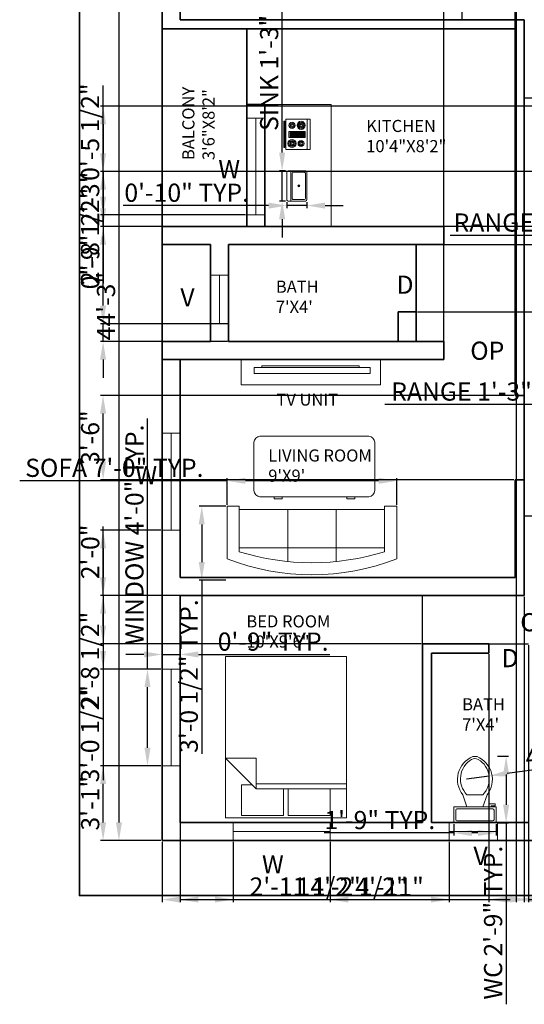
# Model space of a CAD drawing. Units: inches. Extents: x 53076 to 53578, y 41072 to 41816.
# Tile 1 of 4: x 53076 to 53326, y 41072 to 41560. Entities that reach past the tile are written whole.
import ezdxf

# ---------------------------------------------------------------- set-up
doc = ezdxf.new("R2010")
doc.units = ezdxf.units.IN
for name, color, linetype, lineweight in [('A-ANNO-DIMS', 2, 'Continuous', 18), ('A-ANNO-TEXT', 7, 'Continuous', 18), ('A-ANNO-TTLB', 7, 'Continuous', 35), ('A-AREA-IDEN', 7, 'Continuous', 18), ('A-DOOR', 3, 'Continuous', 25), ('A-EQPM', 8, 'Continuous', 18), ('A-FLOR-CASE', 9, 'Continuous', 18), ('A-FLOR-FIXT', 9, 'Continuous', 18), ('A-FURN', 8, 'Continuous', 18), ('A-GLAZ', 4, 'Continuous', 18), ('A-WALL', 7, 'Continuous', 35)]:
    doc.layers.add(name, color=color, linetype=linetype, lineweight=lineweight)
doc.styles.get("Standard").update_dxf_attribs({"font": 'arial.ttf'})
doc.dimstyles.new('ISO-25', dxfattribs={"dimtxt": 9, "dimasz": 9, "dimexe": 1.25, "dimexo": 0.625, "dimtad": 1, "dimdec": 1, "dimrnd": 9, "dimlunit": 3, "dimtxsty": 'Standard', "dimcen": 2.5, "dimadec": 0, "dimazin": 0, "dimtfac": 1, "dimtdec": 1, "dimtmove": 0, "dimatfit": 3, "dimfxl": 1, "dimarcsym": 0})

# ---------------------------------------------------------------- blocks, each defined once
blk = doc.blocks.new('*D2')
at = {"layer": 'A-ANNO-DIMS', "color": 0, "lineweight": -2, "transparency": 16777216}
for p, q in [((53146.18, 41682.66), (53124.21, 41682.66)), ((53125.46, 41673.66), (53125.46, 41161.66)), ((53146.18, 41152.66), (53124.21, 41152.66))]:
    blk.add_line(p, q, dxfattribs=at)
at = {"layer": 'A-ANNO-DIMS', "color": 0, "transparency": 16777216}
for points in [[(53123.96, 41673.66), (53126.96, 41673.66), (53125.46, 41682.66)], [(53123.96, 41161.66), (53126.96, 41161.66), (53125.46, 41152.66)]]:
    blk.add_solid(points, dxfattribs=at)
at = {"layer": 'Defpoints', "color": 0, "transparency": 16777216}
for p in [(53146.81, 41682.66), (53125.46, 41152.66), (53146.81, 41152.66)]:
    blk.add_point(p, dxfattribs=at)
at = {"layer": 'A-ANNO-DIMS', "color": 0, "transparency": 16777216, "insert": (53120.23, 41417.66), "char_height": 9, "attachment_point": 5, "rotation": 90}
blk.add_mtext('44\'-3"', dxfattribs=at)
blk = doc.blocks.new('Range-Oven - 30 in top')
for p, q in [((0, -3), (30, -3)), ((12, -6), (18, -6)), ((13, -20), (13, -6)), ((14, -6), (14, -20)), ((15, -20), (15, -6)), ((16, -6), (16, -20)), ((17, -20), (17, -6)), ((6, -24), (6, -25)), ((8, -25), (8, -24)), ((18, -20), (12, -20)), ((22, -25), (22, -24)), ((24, -24), (24, -25))]:
    blk.add_line(p, q)
for points in [[(0, -24), (0, 0), (30, 0), (30, -24)], [(12, -21), (12, -5), (18, -5), (18, -21)], [(2, -26), (2, -25), (28, -25), (28, -26)]]:
    blk.add_lwpolyline(points, close=True)
for centre, radius in [((6, -9), 4), ((6, -9), 3), ((6, -9), 2), ((6, -9), 1), ((24, -9), 3), ((24, -9), 2), ((24, -9), 1), ((6, -18), 3), ((6, -18), 2), ((6, -18), 1), ((24, -18), 4), ((24, -18), 3), ((24, -18), 2), ((24, -18), 1)]:
    blk.add_circle(centre, radius)
blk = doc.blocks.new('Sink-single - 30 in top')
blk.add_line((-15, -3.999996), (15, -3.999996))
for points in [[(-13.5, 0), (13.5, 0)], [(-15, -18.499996), (-15, -1.5)], [(-13.5, -17.499996), (-13.5, -6.499996)], [(-12.5, -5.499996), (12.5, -5.499996)], [(13.5, -6.499996), (13.5, -17.499996)], [(15, -1.5), (15, -18.499996)], [(12.5, -18.499996), (-12.5, -18.499996)], [(13.5, -19.999996), (-13.5, -19.999996)]]:
    blk.add_lwpolyline(points)
for radius in [1, 0.5]:
    blk.add_circle((0, -11.999996), radius)
for centre, radius, start, end in [((-13.5, -1.5), 1.5, 90, 180), ((-12.5, -6.499996), 1, 90, 180), ((12.5, -6.499996), 1, 0, 90), ((13.5, -1.5), 1.5, 0, 90), ((-13.5, -18.499996), 1.5, 180, 270), ((-12.5, -17.499996), 1, 180, 270), ((12.5, -17.499996), 1, 270, 0), ((13.5, -18.499996), 1.5, 270, 0)]:
    blk.add_arc(centre, radius, start, end)
blk = doc.blocks.new('Sofa - Roundback 7 ft.')
for p, q in [((-12.00002, -32.4421), (-12.00003, -6.5971)), ((11.99997, -32.4421), (11.99998, -6.5971)), ((-36.000027, -34), (-36.000027, -11.4696)), ((-35.999844, -13.3819), (35.9998, -13.3819)), ((35.99998, -34), (35.99998, -11.4696)), ((-36.000027, -32.4421), (35.99998, -32.4421))]:
    blk.add_line(p, q)
for points in [[(-36.000027, -34), (-42.000027, -34), (-42.000027, -8)], [(41.99998, -8), (41.99998, -34), (35.99998, -34)]]:
    blk.add_lwpolyline(points)
for centre, radius, start, end in [((0, -114.25), 114.25, 68.43141, 111.5686), ((-0.00001, -127.1968), 121.1968, 72.72033, 107.2797)]:
    blk.add_arc(centre, radius, start, end)
blk = doc.blocks.new('Desk - 30 x 60 in.')
for p, q in [((-26.999995, 0), (26.999995, 0)), ((-29.999995, -27), (-29.999995, -3)), ((29.999995, -3), (29.999995, -27)), ((26.999995, -30), (-26.999995, -30)), ((-20.000005, -30), (-20.000005, -31)), ((-20.000005, -31), (-16.000005, -31)), ((-16.000005, -31), (-16.000005, -30)), ((15.999995, -31), (15.999995, -30)), ((19.999995, -31), (15.999995, -31)), ((19.999995, -30), (19.999995, -31))]:
    blk.add_line(p, q)
for centre, start, end in [((-26.499995, -3.5), 98.1301, 171.8699), ((26.499995, -3.5), 8.130102, 81.8699), ((-26.499995, -26.5), 188.1301, 261.8699), ((26.499995, -26.5), 278.1301, 351.8699)]:
    blk.add_arc(centre, 3.535534, start, end)
blk = doc.blocks.new('Bed - Queen')
for p, q in [((0, -80.00003), (0, 0)), ((0, 0), (59.99999, 0)), ((59.99999, 0), (59.99999, -80.00003)), ((7.99999, -1.2), (28.79998, -1.2)), ((7.99999, -14.4), (7.99999, -1.2)), ((28.79998, -1.2), (28.79998, -14.4)), ((31.19999, -1.2), (51.99999, -1.2)), ((31.19999, -14.4), (31.19999, -1.2)), ((51.99999, -1.2), (51.99999, -16.4)), ((0, -14.4), (44.8, -14.4)), ((59.99999, -29.6), (44.8, -14.4)), ((44.8, -14.4), (44.8, -29.6)), ((44.8, -16.8), (0, -16.8)), ((51.99999, -16.4), (46.79936, -16.4)), ((44.8, -29.6), (59.99999, -29.6)), ((59.99999, -80.00003), (0, -80.00003))]:
    blk.add_line(p, q)
blk = doc.blocks.new('Toilet - top')
for p, q in [((9.5, -6), (9.5, -2)), ((-10, -8.5), (-8, -8.5)), ((-10, -9.5), (-10, -8.5)), ((-7, -9.5), (-10, -9.5)), ((-8, -8.5), (-8, -8)), ((-7, -8), (-7, -9.5)), ((-4, -8), (-6, -14)), ((4, -8), (6, -14)), ((4, -14), (-4, -14))]:
    blk.add_line(p, q)
blk.add_lwpolyline([(10.5, -8), (10.5, 0), (-10.5, 0), (-10.5, -8)], close=True)
for points in [[(-9.5, -2), (-9.5, -6)], [(8.5, -1), (-8.5, -1)], [(-8.5, -7), (8.5, -7)]]:
    blk.add_lwpolyline(points)
for centre, radius, start, end in [((-8.62, -1.88), 0.884, 81.8699, 188.1301), ((8.62, -1.88), 0.884, 351.8699, 98.1301), ((-8.62, -6.12), 0.884, 171.8699, 278.1301), ((8.62, -6.12), 0.884, 261.8699, 8.1301), ((3.52, -21.58), 12.17, 141.4691, 247.9714), ((4.2, -21.82), 11.33, 136.3677, 238.9468), ((-3.52, -21.58), 12.17, 292.0284, 38.5307), ((-4.2, -21.82), 11.33, 301.053, 43.6321), ((0, -27.88), 4, 245.7318, 294.2682), ((0, -29), 4, 254.8605, 285.1395)]:
    blk.add_arc(centre, radius, start, end)
blk = doc.blocks.new('WIN-48IN')
for p, q in [((0, 48), (9, 48)), ((4.5, 48), (4.5, 0)), ((0, 0), (9, 0))]:
    blk.add_line(p, q)
blk = doc.blocks.new('VENT-24IN')
for p, q in [((0, 9), (0, 0)), ((24, 9), (24, 0)), ((0, 4.5), (24, 4.5))]:
    blk.add_line(p, q)
blk = doc.blocks.new('DOOR-ENTRY-28_5IN')
blk.add_line((0, 0), (28.5, 0))
blk = doc.blocks.new('*D12')
at = {"layer": 'A-ANNO-DIMS', "color": 0, "lineweight": -2, "transparency": 16777216}
for p, q in [((53139.61, 41237.75), (53139.61, 41361.89)), ((53146.18, 41237.75), (53138.36, 41237.75)), ((53139.61, 41198.75), (53139.61, 41228.75)), ((53146.18, 41189.75), (53138.36, 41189.75))]:
    blk.add_line(p, q, dxfattribs=at)
at = {"layer": 'A-ANNO-DIMS', "color": 0, "transparency": 16777216}
for points in [[(53138.11, 41228.75), (53141.11, 41228.75), (53139.61, 41237.75)], [(53138.11, 41198.75), (53141.11, 41198.75), (53139.61, 41189.75)]]:
    blk.add_solid(points, dxfattribs=at)
at = {"layer": 'Defpoints', "color": 0, "transparency": 16777216}
for p in [(53139.61, 41237.75), (53146.81, 41237.75), (53146.81, 41189.75)]:
    blk.add_point(p, dxfattribs=at)
at = {"layer": 'A-ANNO-DIMS', "color": 0, "transparency": 16777216, "insert": (53134.32, 41304.32), "char_height": 9, "attachment_point": 5, "rotation": 90}
blk.add_mtext('WINDOW 4\'-0" TYP.', dxfattribs=at)
blk = doc.blocks.new('*D13')
at = {"layer": 'A-ANNO-DIMS', "color": 0, "lineweight": -2, "transparency": 16777216}
for p, q in [((53137.81, 41244.95), (53128.81, 41244.95)), ((53146.81, 41238.38), (53146.81, 41246.2)), ((53146.81, 41244.95), (53155.81, 41244.95)), ((53155.81, 41238.38), (53155.81, 41246.2)), ((53164.81, 41244.95), (53229.92, 41244.95))]:
    blk.add_line(p, q, dxfattribs=at)
at = {"layer": 'A-ANNO-DIMS', "color": 0, "transparency": 16777216}
for points in [[(53137.81, 41246.45), (53137.81, 41243.45), (53146.81, 41244.95)], [(53164.81, 41246.45), (53164.81, 41243.45), (53155.81, 41244.95)]]:
    blk.add_solid(points, dxfattribs=at)
at = {"layer": 'Defpoints', "color": 0, "transparency": 16777216}
for p in [(53155.81, 41244.95), (53146.81, 41237.75), (53155.81, 41237.75)]:
    blk.add_point(p, dxfattribs=at)
at = {"layer": 'A-ANNO-DIMS', "color": 0, "transparency": 16777216, "insert": (53201.86, 41250.17), "char_height": 9, "attachment_point": 5}
blk.add_mtext('0\'-9" TYP.', dxfattribs=at)
blk = doc.blocks.new('*D14')
at = {"layer": 'A-ANNO-DIMS', "color": 0, "lineweight": -2, "transparency": 16777216}
for p, q in [((53179.09, 41331.04), (53076.3, 41331.04)), ((53179.09, 41319.06), (53179.09, 41332.29)), ((53254.09, 41331.04), (53188.09, 41331.04)), ((53263.09, 41319.06), (53263.09, 41332.29))]:
    blk.add_line(p, q, dxfattribs=at)
at = {"layer": 'A-ANNO-DIMS', "color": 0, "transparency": 16777216}
for points in [[(53188.09, 41332.54), (53188.09, 41329.54), (53179.09, 41331.04)], [(53254.09, 41332.54), (53254.09, 41329.54), (53263.09, 41331.04)]]:
    blk.add_solid(points, dxfattribs=at)
at = {"layer": 'Defpoints', "color": 0, "transparency": 16777216}
for p in [(53179.09, 41331.04), (53179.09, 41318.44), (53263.09, 41318.44)]:
    blk.add_point(p, dxfattribs=at)
at = {"layer": 'A-ANNO-DIMS', "color": 0, "transparency": 16777216, "insert": (53123.19, 41336.32), "char_height": 9, "attachment_point": 5}
blk.add_mtext('SOFA 7\'-0" TYP.', dxfattribs=at)
blk = doc.blocks.new('*D15')
at = {"layer": 'A-ANNO-DIMS', "color": 0, "lineweight": -2, "transparency": 16777216}
for p, q in [((53178.46, 41318.44), (53165.24, 41318.44)), ((53166.49, 41309.44), (53166.49, 41290.77)), ((53178.46, 41281.77), (53165.24, 41281.77)), ((53166.49, 41281.77), (53166.49, 41195.7))]:
    blk.add_line(p, q, dxfattribs=at)
at = {"layer": 'A-ANNO-DIMS', "color": 0, "transparency": 16777216}
for points in [[(53164.99, 41309.44), (53167.99, 41309.44), (53166.49, 41318.44)], [(53164.99, 41290.77), (53167.99, 41290.77), (53166.49, 41281.77)]]:
    blk.add_solid(points, dxfattribs=at)
at = {"layer": 'Defpoints', "color": 0, "transparency": 16777216}
for p in [(53179.09, 41318.44), (53166.49, 41281.77), (53179.09, 41281.77)]:
    blk.add_point(p, dxfattribs=at)
at = {"layer": 'A-ANNO-DIMS', "color": 0, "transparency": 16777216, "insert": (53161.21, 41234.23), "char_height": 9, "attachment_point": 5, "rotation": 90}
blk.add_mtext('3\'-0 1/2" TYP.', dxfattribs=at)
blk = doc.blocks.new('*D18')
at = {"layer": 'A-ANNO-DIMS', "color": 0, "lineweight": -2, "transparency": 16777216}
for p, q in [((53206.33, 41493.74), (53206.33, 41591.64)), ((53207.95, 41484.74), (53205.08, 41484.74)), ((53206.33, 41469.74), (53206.33, 41484.74)), ((53207.95, 41469.74), (53205.08, 41469.74)), ((53206.33, 41460.74), (53206.33, 41451.74))]:
    blk.add_line(p, q, dxfattribs=at)
at = {"layer": 'A-ANNO-DIMS', "color": 0, "transparency": 16777216}
for points in [[(53204.83, 41493.74), (53207.83, 41493.74), (53206.33, 41484.74)], [(53204.83, 41460.74), (53207.83, 41460.74), (53206.33, 41469.74)]]:
    blk.add_solid(points, dxfattribs=at)
at = {"layer": 'Defpoints', "color": 0, "transparency": 16777216}
for p in [(53206.33, 41484.74), (53208.58, 41484.74), (53208.58, 41469.74)]:
    blk.add_point(p, dxfattribs=at)
at = {"layer": 'A-ANNO-DIMS', "color": 0, "transparency": 16777216, "insert": (53201.05, 41547.19), "char_height": 9, "attachment_point": 5, "rotation": 90}
blk.add_mtext('SINK 1\'-3" TYP.', dxfattribs=at)
blk = doc.blocks.new('*D19')
at = {"layer": 'A-ANNO-DIMS', "color": 0, "lineweight": -2, "transparency": 16777216}
for p, q in [((53199.58, 41467.49), (53127.48, 41467.49)), ((53208.58, 41469.11), (53208.58, 41466.24)), ((53218.58, 41467.49), (53208.58, 41467.49)), ((53218.58, 41469.11), (53218.58, 41466.24)), ((53227.58, 41467.49), (53236.58, 41467.49))]:
    blk.add_line(p, q, dxfattribs=at)
at = {"layer": 'A-ANNO-DIMS', "color": 0, "transparency": 16777216}
for points in [[(53199.58, 41468.99), (53199.58, 41465.99), (53208.58, 41467.49)], [(53227.58, 41468.99), (53227.58, 41465.99), (53218.58, 41467.49)]]:
    blk.add_solid(points, dxfattribs=at)
at = {"layer": 'Defpoints', "color": 0, "transparency": 16777216}
for p in [(53208.58, 41469.74), (53208.58, 41467.49), (53218.58, 41469.74)]:
    blk.add_point(p, dxfattribs=at)
at = {"layer": 'A-ANNO-DIMS', "color": 0, "transparency": 16777216, "insert": (53159.03, 41472.71), "char_height": 9, "attachment_point": 5}
blk.add_mtext('0\'-10" TYP.', dxfattribs=at)
blk = doc.blocks.new('*D20')
at = {"layer": 'A-ANNO-DIMS', "color": 0, "lineweight": -2, "transparency": 16777216}
for p, q in [((53371.57, 41452.66), (53289.65, 41452.66)), ((53371.57, 41456.53), (53371.57, 41451.41)), ((53392.57, 41452.66), (53380.57, 41452.66)), ((53401.57, 41456.53), (53401.57, 41451.41))]:
    blk.add_line(p, q, dxfattribs=at)
at = {"layer": 'A-ANNO-DIMS', "color": 0, "transparency": 16777216}
for points in [[(53380.57, 41454.16), (53380.57, 41451.16), (53371.57, 41452.66)], [(53392.57, 41454.16), (53392.57, 41451.16), (53401.57, 41452.66)]]:
    blk.add_solid(points, dxfattribs=at)
at = {"layer": 'Defpoints', "color": 0, "transparency": 16777216}
for p in [(53371.57, 41457.16), (53371.57, 41452.66), (53401.57, 41457.16)]:
    blk.add_point(p, dxfattribs=at)
at = {"layer": 'A-ANNO-DIMS', "color": 0, "transparency": 16777216, "insert": (53326.11, 41457.93), "char_height": 9, "attachment_point": 5}
blk.add_mtext('RANGE 2\'-6"', dxfattribs=at)
blk = doc.blocks.new('*D22')
at = {"layer": 'A-ANNO-DIMS', "color": 0, "lineweight": -2, "transparency": 16777216}
for p, q in [((53379.04, 41367.23), (53379.04, 41370.11)), ((53394.04, 41367.23), (53394.04, 41370.11)), ((53370.04, 41368.86), (53257.19, 41368.86)), ((53394.04, 41368.86), (53379.04, 41368.86)), ((53403.04, 41368.86), (53412.04, 41368.86))]:
    blk.add_line(p, q, dxfattribs=at)
at = {"layer": 'A-ANNO-DIMS', "color": 0, "transparency": 16777216}
for points in [[(53370.04, 41370.36), (53370.04, 41367.36), (53379.04, 41368.86)], [(53403.04, 41370.36), (53403.04, 41367.36), (53394.04, 41368.86)]]:
    blk.add_solid(points, dxfattribs=at)
at = {"layer": 'Defpoints', "color": 0, "transparency": 16777216}
for p in [(53379.04, 41368.86), (53379.04, 41366.61), (53394.04, 41366.61)]:
    blk.add_point(p, dxfattribs=at)
at = {"layer": 'A-ANNO-DIMS', "color": 0, "transparency": 16777216, "insert": (53309.12, 41374.14), "char_height": 9, "attachment_point": 5}
blk.add_mtext('RANGE 1\'-3" TYP.', dxfattribs=at)
blk = doc.blocks.new('*D30')
at = {"layer": 'A-ANNO-DIMS', "color": 0, "lineweight": -2, "transparency": 16777216}
for p, q in [((53312.97, 41194.48), (53318.55, 41194.48)), ((53317.3, 41185.48), (53317.3, 41170.44)), ((53312.97, 41161.44), (53318.55, 41161.44)), ((53317.3, 41161.44), (53317.3, 41071.52))]:
    blk.add_line(p, q, dxfattribs=at)
at = {"layer": 'A-ANNO-DIMS', "color": 0, "transparency": 16777216}
for points in [[(53315.8, 41185.48), (53318.8, 41185.48), (53317.3, 41194.48)], [(53315.8, 41170.44), (53318.8, 41170.44), (53317.3, 41161.44)]]:
    blk.add_solid(points, dxfattribs=at)
at = {"layer": 'Defpoints', "color": 0, "transparency": 16777216}
for p in [(53312.34, 41194.48), (53312.34, 41161.44), (53317.3, 41161.44)]:
    blk.add_point(p, dxfattribs=at)
at = {"layer": 'A-ANNO-DIMS', "color": 0, "transparency": 16777216, "insert": (53312.02, 41111.98), "char_height": 9, "attachment_point": 5, "rotation": 90}
blk.add_mtext('WC 2\'-9" TYP.', dxfattribs=at)
blk = doc.blocks.new('*D31')
at = {"layer": 'A-ANNO-DIMS', "color": 0, "lineweight": -2, "transparency": 16777216}
for p, q in [((53291.34, 41160.81), (53291.34, 41155.23)), ((53312.34, 41160.81), (53312.34, 41155.23)), ((53291.34, 41156.48), (53227.08, 41156.48)), ((53303.34, 41156.48), (53300.34, 41156.48))]:
    blk.add_line(p, q, dxfattribs=at)
at = {"layer": 'A-ANNO-DIMS', "color": 0, "transparency": 16777216}
for points in [[(53300.34, 41157.98), (53300.34, 41154.98), (53291.34, 41156.48)], [(53303.34, 41157.98), (53303.34, 41154.98), (53312.34, 41156.48)]]:
    blk.add_solid(points, dxfattribs=at)
at = {"layer": 'Defpoints', "color": 0, "transparency": 16777216}
for p in [(53291.34, 41161.44), (53312.34, 41161.44), (53291.34, 41156.48)]:
    blk.add_point(p, dxfattribs=at)
at = {"layer": 'A-ANNO-DIMS', "color": 0, "transparency": 16777216, "insert": (53254.71, 41161.7), "char_height": 9, "attachment_point": 5}
blk.add_mtext('1\'-9" TYP.', dxfattribs=at)
blk = doc.blocks.new('*D36')
at = {"layer": 'A-ANNO-DIMS', "color": 0, "lineweight": -2, "transparency": 16777216}
for p, q in [((53155.18, 41274.16), (53116.36, 41274.16)), ((53117.61, 41265.16), (53117.61, 41246.75)), ((53146.18, 41237.75), (53116.36, 41237.75)), ((53117.61, 41237.75), (53117.61, 41182.61))]:
    blk.add_line(p, q, dxfattribs=at)
at = {"layer": 'A-ANNO-DIMS', "color": 0, "transparency": 16777216}
for points in [[(53116.11, 41265.16), (53119.11, 41265.16), (53117.61, 41274.16)], [(53116.11, 41246.75), (53119.11, 41246.75), (53117.61, 41237.75)]]:
    blk.add_solid(points, dxfattribs=at)
at = {"layer": 'Defpoints', "color": 0, "transparency": 16777216}
for p in [(53155.81, 41274.16), (53117.61, 41237.75), (53146.81, 41237.75)]:
    blk.add_point(p, dxfattribs=at)
at = {"layer": 'A-ANNO-DIMS', "color": 0, "transparency": 16777216, "insert": (53112.32, 41205.68), "char_height": 9, "attachment_point": 5, "rotation": 90}
blk.add_mtext('3\'-0 1/2"', dxfattribs=at)
blk = doc.blocks.new('*D42')
at = {"layer": 'A-ANNO-DIMS', "color": 0, "lineweight": -2, "transparency": 16777216}
for p, q in [((53146.81, 41152.03), (53146.81, 41122.21)), ((53182.09, 41152.03), (53182.09, 41122.21)), ((53155.81, 41123.46), (53173.09, 41123.46)), ((53182.09, 41123.46), (53244.38, 41123.46))]:
    blk.add_line(p, q, dxfattribs=at)
at = {"layer": 'A-ANNO-DIMS', "color": 0, "transparency": 16777216}
for points in [[(53155.81, 41124.96), (53155.81, 41121.96), (53146.81, 41123.46)], [(53173.09, 41124.96), (53173.09, 41121.96), (53182.09, 41123.46)]]:
    blk.add_solid(points, dxfattribs=at)
at = {"layer": 'Defpoints', "color": 0, "transparency": 16777216}
for p in [(53146.81, 41152.66), (53182.09, 41152.66), (53182.09, 41123.46)]:
    blk.add_point(p, dxfattribs=at)
at = {"layer": 'A-ANNO-DIMS', "color": 0, "transparency": 16777216, "insert": (53217.73, 41128.73), "char_height": 9, "attachment_point": 5}
blk.add_mtext('2\'-11 1/2"', dxfattribs=at)
blk = doc.blocks.new('*D43')
at = {"layer": 'A-ANNO-DIMS', "color": 0, "lineweight": -2, "transparency": 16777216}
for p, q in [((53230.09, 41152.03), (53230.09, 41122.21)), ((53289.01, 41152.03), (53289.01, 41122.21)), ((53239.09, 41123.46), (53280.01, 41123.46))]:
    blk.add_line(p, q, dxfattribs=at)
at = {"layer": 'A-ANNO-DIMS', "color": 0, "transparency": 16777216}
for points in [[(53239.09, 41124.96), (53239.09, 41121.96), (53230.09, 41123.46)], [(53280.01, 41124.96), (53280.01, 41121.96), (53289.01, 41123.46)]]:
    blk.add_solid(points, dxfattribs=at)
at = {"layer": 'Defpoints', "color": 0, "transparency": 16777216}
for p in [(53230.09, 41152.66), (53289.01, 41152.66), (53289.01, 41123.46)]:
    blk.add_point(p, dxfattribs=at)
at = {"layer": 'A-ANNO-DIMS', "color": 0, "transparency": 16777216, "insert": (53259.55, 41128.6), "char_height": 9, "attachment_point": 5}
blk.add_mtext('4\'-11"', dxfattribs=at)
blk = doc.blocks.new('*D46')
at = {"layer": 'A-ANNO-DIMS', "color": 0, "lineweight": -2, "transparency": 16777216}
for p, q in [((53146.18, 41306.6), (53116.36, 41306.6)), ((53117.61, 41297.6), (53117.61, 41283.16)), ((53155.18, 41274.16), (53116.36, 41274.16)), ((53117.61, 41274.16), (53117.61, 41218.86))]:
    blk.add_line(p, q, dxfattribs=at)
at = {"layer": 'A-ANNO-DIMS', "color": 0, "transparency": 16777216}
for points in [[(53116.11, 41297.6), (53119.11, 41297.6), (53117.61, 41306.6)], [(53116.11, 41283.16), (53119.11, 41283.16), (53117.61, 41274.16)]]:
    blk.add_solid(points, dxfattribs=at)
at = {"layer": 'Defpoints', "color": 0, "transparency": 16777216}
for p in [(53146.81, 41306.6), (53117.61, 41274.16), (53155.81, 41274.16)]:
    blk.add_point(p, dxfattribs=at)
at = {"layer": 'A-ANNO-DIMS', "color": 0, "transparency": 16777216, "insert": (53112.33, 41242.01), "char_height": 9, "attachment_point": 5, "rotation": 90}
blk.add_mtext('2\'-8 1/2"', dxfattribs=at)
blk = doc.blocks.new('*D47')
at = {"layer": 'A-ANNO-DIMS', "color": 0, "lineweight": -2, "transparency": 16777216}
for p, q in [((53146.18, 41189.75), (53116.36, 41189.75)), ((53117.61, 41161.66), (53117.61, 41180.75)), ((53146.18, 41152.66), (53116.36, 41152.66))]:
    blk.add_line(p, q, dxfattribs=at)
at = {"layer": 'A-ANNO-DIMS', "color": 0, "transparency": 16777216}
for points in [[(53116.11, 41180.75), (53119.11, 41180.75), (53117.61, 41189.75)], [(53116.11, 41161.66), (53119.11, 41161.66), (53117.61, 41152.66)]]:
    blk.add_solid(points, dxfattribs=at)
at = {"layer": 'Defpoints', "color": 0, "transparency": 16777216}
for p in [(53117.61, 41189.75), (53146.81, 41189.75), (53146.81, 41152.66)]:
    blk.add_point(p, dxfattribs=at)
at = {"layer": 'A-ANNO-DIMS', "color": 0, "transparency": 16777216, "insert": (53112.38, 41171.2), "char_height": 9, "attachment_point": 5, "rotation": 90}
blk.add_mtext('3\'-1"', dxfattribs=at)
blk = doc.blocks.new('*D50')
at = {"layer": 'A-ANNO-DIMS', "color": 0, "lineweight": -2, "transparency": 16777216}
for p, q in [((53117.61, 41471.84), (53117.61, 41526.99)), ((53188.18, 41462.84), (53116.36, 41462.84)), ((53117.61, 41457.16), (53117.61, 41462.84)), ((53188.18, 41457.16), (53116.36, 41457.16)), ((53117.61, 41448.16), (53117.61, 41439.16))]:
    blk.add_line(p, q, dxfattribs=at)
at = {"layer": 'A-ANNO-DIMS', "color": 0, "transparency": 16777216}
for points in [[(53116.11, 41471.84), (53119.11, 41471.84), (53117.61, 41462.84)], [(53116.11, 41448.16), (53119.11, 41448.16), (53117.61, 41457.16)]]:
    blk.add_solid(points, dxfattribs=at)
at = {"layer": 'Defpoints', "color": 0, "transparency": 16777216}
for p in [(53117.61, 41462.84), (53188.81, 41462.84), (53188.81, 41457.16)]:
    blk.add_point(p, dxfattribs=at)
at = {"layer": 'A-ANNO-DIMS', "color": 0, "transparency": 16777216, "insert": (53112.33, 41503.92), "char_height": 9, "attachment_point": 5, "rotation": 90}
blk.add_mtext('0\'-5 1/2"', dxfattribs=at)
blk = doc.blocks.new('*D51')
at = {"layer": 'A-ANNO-DIMS', "color": 0, "lineweight": -2, "transparency": 16777216}
for p, q in [((53117.61, 41417.95), (53117.61, 41452.12)), ((53179.18, 41408.95), (53116.36, 41408.95)), ((53117.61, 41400.16), (53117.61, 41408.95)), ((53179.18, 41400.16), (53116.36, 41400.16)), ((53117.61, 41391.16), (53117.61, 41382.16))]:
    blk.add_line(p, q, dxfattribs=at)
at = {"layer": 'A-ANNO-DIMS', "color": 0, "transparency": 16777216}
for points in [[(53116.11, 41417.95), (53119.11, 41417.95), (53117.61, 41408.95)], [(53116.11, 41391.16), (53119.11, 41391.16), (53117.61, 41400.16)]]:
    blk.add_solid(points, dxfattribs=at)
at = {"layer": 'Defpoints', "color": 0, "transparency": 16777216}
for p in [(53117.61, 41408.95), (53179.81, 41408.95), (53179.81, 41400.16)]:
    blk.add_point(p, dxfattribs=at)
at = {"layer": 'A-ANNO-DIMS', "color": 0, "transparency": 16777216, "insert": (53112.39, 41439.54), "char_height": 9, "attachment_point": 5, "rotation": 90}
blk.add_mtext('0\'-9"', dxfattribs=at)
blk = doc.blocks.new('*D55')
at = {"layer": 'A-ANNO-DIMS', "color": 0, "lineweight": -2, "transparency": 16777216}
for p, q in [((53322.2, 41589.03), (53322.2, 41122.21)), ((53343.31, 41584.53), (53343.31, 41122.21)), ((53331.2, 41123.46), (53334.31, 41123.46)), ((53343.31, 41123.46), (53376.63, 41123.46))]:
    blk.add_line(p, q, dxfattribs=at)
at = {"layer": 'A-ANNO-DIMS', "color": 0, "transparency": 16777216}
for points in [[(53331.2, 41124.96), (53331.2, 41121.96), (53322.2, 41123.46)], [(53334.31, 41124.96), (53334.31, 41121.96), (53343.31, 41123.46)]]:
    blk.add_solid(points, dxfattribs=at)
at = {"layer": 'Defpoints', "color": 0, "transparency": 16777216}
for p in [(53322.2, 41589.66), (53343.31, 41585.16), (53343.31, 41123.46)]:
    blk.add_point(p, dxfattribs=at)
at = {"layer": 'A-ANNO-DIMS', "color": 0, "transparency": 16777216, "insert": (53364.47, 41128.68), "char_height": 9, "attachment_point": 5}
blk.add_mtext('1\'-9"', dxfattribs=at)
blk = doc.blocks.new('*D57')
at = {"layer": 'A-ANNO-DIMS', "color": 0, "lineweight": -2, "transparency": 16777216}
for p, q in [((53321.18, 41373.39), (53116.36, 41373.39)), ((53117.61, 41340.53), (53117.61, 41364.39)), ((53321.18, 41331.53), (53116.36, 41331.53))]:
    blk.add_line(p, q, dxfattribs=at)
at = {"layer": 'A-ANNO-DIMS', "color": 0, "transparency": 16777216}
for points in [[(53116.11, 41364.39), (53119.11, 41364.39), (53117.61, 41373.39)], [(53116.11, 41340.53), (53119.11, 41340.53), (53117.61, 41331.53)]]:
    blk.add_solid(points, dxfattribs=at)
at = {"layer": 'Defpoints', "color": 0, "transparency": 16777216}
for p in [(53117.61, 41373.39), (53321.81, 41373.39), (53321.81, 41331.53)]:
    blk.add_point(p, dxfattribs=at)
at = {"layer": 'A-ANNO-DIMS', "color": 0, "transparency": 16777216, "insert": (53112.38, 41352.46), "char_height": 9, "attachment_point": 5, "rotation": 90}
blk.add_mtext('3\'-6"', dxfattribs=at)
blk = doc.blocks.new('*D58')
at = {"layer": 'A-ANNO-DIMS', "color": 0, "lineweight": -2, "transparency": 16777216}
for p, q in [((53273.43, 41448.16), (53513.26, 41448.16)), ((53512.01, 41439.16), (53512.01, 41423.85)), ((53273.43, 41414.85), (53513.26, 41414.85)), ((53512.01, 41414.85), (53512.01, 41359.55))]:
    blk.add_line(p, q, dxfattribs=at)
at = {"layer": 'A-ANNO-DIMS', "color": 0, "transparency": 16777216}
for points in [[(53510.51, 41439.16), (53513.51, 41439.16), (53512.01, 41448.16)], [(53510.51, 41423.85), (53513.51, 41423.85), (53512.01, 41414.85)]]:
    blk.add_solid(points, dxfattribs=at)
at = {"layer": 'Defpoints', "color": 0, "transparency": 16777216}
for p in [(53272.81, 41448.16), (53272.81, 41414.85), (53512.01, 41414.85)]:
    blk.add_point(p, dxfattribs=at)
at = {"layer": 'A-ANNO-DIMS', "color": 0, "transparency": 16777216, "insert": (53506.73, 41382.7), "char_height": 9, "attachment_point": 5, "rotation": 90}
blk.add_mtext('2\'-9 1/2"', dxfattribs=at)
blk = doc.blocks.new('*D59')
at = {"layer": 'A-ANNO-DIMS', "color": 0, "lineweight": -2, "transparency": 16777216}
for p, q in [((53117.61, 41274.16), (53117.61, 41308.48)), ((53275.18, 41274.16), (53116.36, 41274.16)), ((53117.61, 41259.16), (53117.61, 41265.16)), ((53275.18, 41250.16), (53116.36, 41250.16))]:
    blk.add_line(p, q, dxfattribs=at)
at = {"layer": 'A-ANNO-DIMS', "color": 0, "transparency": 16777216}
for points in [[(53116.11, 41265.16), (53119.11, 41265.16), (53117.61, 41274.16)], [(53116.11, 41259.16), (53119.11, 41259.16), (53117.61, 41250.16)]]:
    blk.add_solid(points, dxfattribs=at)
at = {"layer": 'Defpoints', "color": 0, "transparency": 16777216}
for p in [(53117.61, 41274.16), (53275.81, 41274.16), (53275.81, 41250.16)]:
    blk.add_point(p, dxfattribs=at)
at = {"layer": 'A-ANNO-DIMS', "color": 0, "transparency": 16777216, "insert": (53112.39, 41295.82), "char_height": 9, "attachment_point": 5, "rotation": 90}
blk.add_mtext('2\'-0"', dxfattribs=at)
blk = doc.blocks.new('*D60')
at = {"layer": 'A-ANNO-DIMS', "color": 0, "lineweight": -2, "transparency": 16777216}
for p, q in [((53286.43, 41391.78), (53286.43, 41713.11)), ((53295.43, 41711.86), (53312.81, 41711.86)), ((53321.81, 41374.01), (53321.81, 41713.11)), ((53321.81, 41711.86), (53384.1, 41711.86))]:
    blk.add_line(p, q, dxfattribs=at)
at = {"layer": 'A-ANNO-DIMS', "color": 0, "transparency": 16777216}
for points in [[(53295.43, 41713.36), (53295.43, 41710.36), (53286.43, 41711.86)], [(53312.81, 41713.36), (53312.81, 41710.36), (53321.81, 41711.86)]]:
    blk.add_solid(points, dxfattribs=at)
at = {"layer": 'Defpoints', "color": 0, "transparency": 16777216}
for p in [(53321.81, 41711.86), (53286.43, 41391.16), (53321.81, 41373.39)]:
    blk.add_point(p, dxfattribs=at)
at = {"layer": 'A-ANNO-DIMS', "color": 0, "transparency": 16777216, "insert": (53357.45, 41717.13), "char_height": 9, "attachment_point": 5}
blk.add_mtext('2\'-11 1/2"', dxfattribs=at)
blk = doc.blocks.new('*D66')
at = {"layer": 'A-ANNO-DIMS', "color": 0, "lineweight": -2, "transparency": 16777216}
for p, q in [((53363.18, 41484.39), (53116.36, 41484.39)), ((53117.61, 41466.16), (53117.61, 41475.39)), ((53363.18, 41457.16), (53116.36, 41457.16))]:
    blk.add_line(p, q, dxfattribs=at)
at = {"layer": 'A-ANNO-DIMS', "color": 0, "transparency": 16777216}
for points in [[(53116.11, 41475.39), (53119.11, 41475.39), (53117.61, 41484.39)], [(53116.11, 41466.16), (53119.11, 41466.16), (53117.61, 41457.16)]]:
    blk.add_solid(points, dxfattribs=at)
at = {"layer": 'Defpoints', "color": 0, "transparency": 16777216}
for p in [(53117.61, 41484.39), (53363.81, 41484.39), (53363.81, 41457.16)]:
    blk.add_point(p, dxfattribs=at)
at = {"layer": 'A-ANNO-DIMS', "color": 0, "transparency": 16777216, "insert": (53112.38, 41470.77), "char_height": 9, "attachment_point": 5, "rotation": 90}
blk.add_mtext('2\'-3"', dxfattribs=at)
blk = doc.blocks.new('*D68')
at = {"layer": 'A-ANNO-DIMS', "color": 0, "lineweight": -2, "transparency": 16777216}
for p, q in [((53155.81, 41273.53), (53155.81, 41122.21)), ((53326.31, 41273.53), (53326.31, 41122.21)), ((53164.81, 41123.46), (53317.31, 41123.46))]:
    blk.add_line(p, q, dxfattribs=at)
at = {"layer": 'A-ANNO-DIMS', "color": 0, "transparency": 16777216}
for points in [[(53164.81, 41124.96), (53164.81, 41121.96), (53155.81, 41123.46)], [(53317.31, 41124.96), (53317.31, 41121.96), (53326.31, 41123.46)]]:
    blk.add_solid(points, dxfattribs=at)
at = {"layer": 'Defpoints', "color": 0, "transparency": 16777216}
for p in [(53155.81, 41274.16), (53326.31, 41274.16), (53326.31, 41123.46)]:
    blk.add_point(p, dxfattribs=at)
at = {"layer": 'A-ANNO-DIMS', "color": 0, "transparency": 16777216, "insert": (53241.06, 41128.73), "char_height": 9, "attachment_point": 5}
blk.add_mtext('14\'-2 1/2"', dxfattribs=at)
blk = doc.blocks.new('*D69')
at = {"layer": 'A-ANNO-DIMS', "color": 0, "lineweight": -2, "transparency": 16777216}
for p, q in [((53328.31, 41249.53), (53328.31, 41122.21)), ((53308.69, 41245.03), (53308.69, 41122.21)), ((53317.69, 41123.46), (53319.31, 41123.46)), ((53328.31, 41123.46), (53382.6, 41123.46))]:
    blk.add_line(p, q, dxfattribs=at)
at = {"layer": 'A-ANNO-DIMS', "color": 0, "transparency": 16777216}
for points in [[(53317.69, 41124.96), (53317.69, 41121.96), (53308.69, 41123.46)], [(53319.31, 41124.96), (53319.31, 41121.96), (53328.31, 41123.46)]]:
    blk.add_solid(points, dxfattribs=at)
at = {"layer": 'Defpoints', "color": 0, "transparency": 16777216}
for p in [(53328.31, 41250.16), (53308.69, 41245.66), (53328.31, 41123.46)]:
    blk.add_point(p, dxfattribs=at)
at = {"layer": 'A-ANNO-DIMS', "color": 0, "transparency": 16777216, "insert": (53359.96, 41128.73), "char_height": 9, "attachment_point": 5}
blk.add_mtext('1\'-7 1/2"', dxfattribs=at)
blk = doc.blocks.new('*D70')
at = {"layer": 'A-ANNO-DIMS', "color": 0, "lineweight": -2, "transparency": 16777216}
for p, q in [((53410.23, 41516.86), (53116.36, 41516.86)), ((53117.61, 41507.86), (53117.61, 41493.39)), ((53410.23, 41484.39), (53116.36, 41484.39)), ((53117.61, 41484.39), (53117.61, 41429.09))]:
    blk.add_line(p, q, dxfattribs=at)
at = {"layer": 'A-ANNO-DIMS', "color": 0, "transparency": 16777216}
for points in [[(53116.11, 41507.86), (53119.11, 41507.86), (53117.61, 41516.86)], [(53116.11, 41493.39), (53119.11, 41493.39), (53117.61, 41484.39)]]:
    blk.add_solid(points, dxfattribs=at)
at = {"layer": 'Defpoints', "color": 0, "transparency": 16777216}
for p in [(53410.86, 41516.86), (53117.61, 41484.39), (53410.86, 41484.39)]:
    blk.add_point(p, dxfattribs=at)
at = {"layer": 'A-ANNO-DIMS', "color": 0, "transparency": 16777216, "insert": (53112.33, 41452.24), "char_height": 9, "attachment_point": 5, "rotation": 90}
blk.add_mtext('2\'-8 1/2"', dxfattribs=at)
blk = doc.blocks.new('*D74')
at = {"layer": 'A-ANNO-DIMS', "color": 0, "lineweight": -2, "transparency": 16777216}
for p, q in [((53407.43, 41198.01), (53317.79, 41185.96)), ((53297.64, 41183.25), (53308.87, 41184.76))]:
    blk.add_line(p, q, dxfattribs=at)
at = {"layer": 'A-ANNO-DIMS', "color": 0, "transparency": 16777216}
blk.add_solid([(53317.59, 41187.45), (53317.99, 41184.48), (53308.87, 41184.76)], dxfattribs=at)
at = {"layer": 'Defpoints', "color": 0, "transparency": 16777216}
for p in [(53308.87, 41184.76), (53297.64, 41183.25)]:
    blk.add_point(p, dxfattribs=at)
at = {"layer": 'A-ANNO-DIMS', "color": 0, "transparency": 16777216, "insert": (53366.37, 41197.82), "char_height": 9, "attachment_point": 5, "rotation": 7.6564}
blk.add_mtext('4X R0\'-11 1/2"', dxfattribs=at)

msp = doc.modelspace()

# ---------------------------------------------------------------- linework, layer by layer
at = {"layer": 'A-ANNO-TTLB'}
msp.add_lwpolyline([(53105.85, 41713.9), (53500.98, 41713.9), (53500.98, 41125.46), (53105.85, 41125.46)], close=True, dxfattribs=at)
at = {"layer": 'A-DOOR'}
for p, q in [((53295.31, 41585.16), (53295.31, 41559.66)), ((53286.43, 41448.16), (53321.81, 41448.16)), ((53275.81, 41250.16), (53275.81, 41274.16)), ((53308.69, 41250.16), (53328.31, 41250.16))]:
    msp.add_line(p, q, dxfattribs=at)
at = {"layer": 'A-EQPM'}
for p, q in [((53196.25, 41387.18), (53196.25, 41388.13)), ((53196.25, 41388.13), (53244.42, 41388.13)), ((53244.42, 41388.13), (53244.42, 41387.18))]:
    msp.add_line(p, q, dxfattribs=at)
msp.add_lwpolyline([(53192.5, 41387.18), (53249.95, 41387.18), (53249.95, 41384.17), (53192.5, 41384.17)], close=True, dxfattribs=at)
at = {"layer": 'A-FLOR-CASE'}
for p, q in [((53197.81, 41517.63), (53230.64, 41517.63)), ((53230.64, 41517.63), (53230.64, 41457.16)), ((53185.97, 41391.16), (53185.97, 41378.63)), ((53255.14, 41378.63), (53255.14, 41391.16)), ((53185.97, 41378.63), (53255.14, 41378.63))]:
    msp.add_line(p, q, dxfattribs=at)
at = {"layer": 'A-WALL'}
for p, q in [((53146.81, 41152.66), (53146.81, 41682.66)), ((53155.81, 41559.66), (53155.81, 41673.66)), ((53146.81, 41555.16), (53321.81, 41555.16)), ((53155.81, 41559.66), (53326.31, 41559.66)), ((53188.81, 41457.16), (53188.81, 41555.16)), ((53321.81, 41373.39), (53321.81, 41555.16)), ((53326.31, 41283.16), (53326.31, 41559.66)), ((53188.81, 41517.63), (53197.81, 41517.63)), ((53197.81, 41457.16), (53197.81, 41517.63)), ((53146.81, 41457.16), (53286.43, 41457.16)), ((53286.43, 41457.16), (53286.43, 41448.16)), ((53146.81, 41448.16), (53170.81, 41448.16)), ((53170.81, 41400.16), (53170.81, 41448.16)), ((53179.81, 41400.16), (53179.81, 41448.16)), ((53179.81, 41448.16), (53286.43, 41448.16)), ((53272.81, 41400.16), (53272.81, 41448.16)), ((53263.81, 41400.16), (53263.81, 41414.85)), ((53263.81, 41414.85), (53272.81, 41414.85)), ((53146.81, 41400.16), (53170.81, 41400.16)), ((53179.81, 41400.16), (53286.43, 41400.16)), ((53286.43, 41400.16), (53286.43, 41391.16)), ((53146.81, 41391.16), (53286.43, 41391.16)), ((53155.81, 41283.16), (53155.81, 41391.16)), ((53321.81, 41373.39), (53326.31, 41373.39)), ((53321.81, 41283.16), (53321.81, 41331.53)), ((53321.81, 41331.53), (53326.31, 41331.53)), ((53155.81, 41283.16), (53286.43, 41283.16)), ((53286.43, 41283.16), (53321.81, 41283.16)), ((53326.31, 41283.16), (53326.31, 41274.16)), ((53155.81, 41161.66), (53155.81, 41274.16)), ((53155.81, 41274.16), (53286.43, 41274.16)), ((53286.43, 41274.16), (53326.31, 41274.16)), ((53275.81, 41161.66), (53275.81, 41250.16)), ((53308.69, 41250.16), (53275.81, 41250.16)), ((53308.69, 41250.16), (53308.69, 41245.66)), ((53280.31, 41161.66), (53280.31, 41245.66)), ((53308.69, 41245.66), (53280.31, 41245.66)), ((53275.81, 41161.66), (53155.81, 41161.66)), ((53328.31, 41161.66), (53280.31, 41161.66)), ((53482.81, 41152.66), (53146.81, 41152.66))]:
    msp.add_line(p, q, dxfattribs=at)

# ---------------------------------------------------------------- block references
at = {"layer": 'A-DOOR'}
for p in [(53326.31, 41520.92), (53326.31, 41313.66)]:
    msp.add_blockref('DOOR-ENTRY-28_5IN', p, dxfattribs=at)
at = {"layer": 'A-EQPM', "xscale": 0.5, "yscale": 0.5, "rotation": 270}
msp.add_blockref('Range-Oven - 30 in top', (53220.22, 41510.28), dxfattribs=at)
at = {"layer": 'A-FLOR-FIXT', "xscale": 0.5, "yscale": 0.5, "rotation": 89.99999999999999}
msp.add_blockref('Sink-single - 30 in top', (53208.58, 41477.24), dxfattribs=at)
at = {"layer": 'A-FLOR-FIXT', "rotation": 180}
msp.add_blockref('Toilet - top', (53301.84, 41161.44), dxfattribs=at)
at = {"layer": 'A-FURN'}
msp.add_blockref('Desk - 30 x 60 in.', (53222.3, 41353.17), dxfattribs=at)
at = {"layer": 'A-FURN', "rotation": 180}
for name, p in [('Sofa - Roundback 7 ft.', (53221.09, 41284.44)), ('Bed - Queen', (53238.18, 41163.96))]:
    msp.add_blockref(name, p, dxfattribs=at)
at = {"layer": 'A-GLAZ'}
for p in [(53188.81, 41462.84), (53146.81, 41306.6), (53146.81, 41189.75)]:
    msp.add_blockref('WIN-48IN', p, dxfattribs=at)
for name, p, rotation in [('VENT-24IN', (53179.81, 41408.95), 89.99999999998097), ('WIN-48IN', (53182.09, 41161.66), 269.9999999999968), ('VENT-24IN', (53313.01, 41161.66), 180)]:
    msp.add_blockref(name, p, dxfattribs=dict(at, rotation=rotation))

# ---------------------------------------------------------------- texts
at = {"layer": 'A-ANNO-TEXT', "attachment_point": 1}
for s, width, insert, char_height in [('W ', 6.4326, (53174.7, 41490.05), 9), ('D ', 6.4326, (53262.98, 41432.78), 9), ('V ', 6.4326, (53155.89, 41426.51), 9), ('OP ', 9, (53299.54, 41400.04), 9), ('TV UNIT', 85.6025, (53203.5, 41374.33), 6), ('W ', 6.4326, (53133.62, 41338.37), 9), ('OP ', 6.4326, (53324.32, 41265.45), 9), ('D ', 6.4326, (53315.03, 41247.65), 9), ('W ', 6.4326, (53196.33, 41145.4), 9), ('V ', 6.4326, (53301.11, 41149.66), 9)]:
    msp.add_mtext_dynamic_manual_height_columns(s, width=width, gutter_width=12.5, heights=[0], dxfattribs=dict(at, insert=insert, char_height=char_height))
at = {"layer": 'A-AREA-IDEN', "insert": (53156.87, 41490.05), "char_height": 6, "attachment_point": 1, "rotation": 90}
msp.add_mtext_dynamic_manual_height_columns('BALCONY\\P3\'6"X8\'2"', width=85.6025, gutter_width=12.5, heights=[0], dxfattribs=at)
at = {"layer": 'A-AREA-IDEN', "char_height": 6, "attachment_point": 1}
for s, insert in [('KITCHEN\\P10\'4"X8\'2"', (53247.99, 41509.98)), ("BATH\\P7'X4'", (53203.2, 41430.29)), ("LIVING ROOM\\P9'X9'", (53199.45, 41346.61)), ('BED ROOM\\P10\'X9\'6"', (53188.61, 41264.37)), ("BATH\\P7'X4'", (53295.51, 41223.26))]:
    msp.add_mtext_dynamic_manual_height_columns(s, width=85.6025, gutter_width=12.5, heights=[0], dxfattribs=dict(at, insert=insert))

# ---------------------------------------------------------------- dimensions: what is measured, and where the dimension line sits
at = {"layer": 'A-ANNO-DIMS'}
for base, p1, p2, picture, middle in [((53321.81, 41711.86), (53286.43, 41391.16), (53321.81, 41373.39), '*D60', (53357.45, 41717.13)), ((53343.31, 41123.46), (53322.2, 41589.66), (53343.31, 41585.16), '*D55', (53364.47, 41128.68)), ((53326.31, 41123.46), (53155.81, 41274.16), (53326.31, 41274.16), '*D68', (53241.06, 41128.73)), ((53328.31, 41123.46), (53308.69, 41245.66), (53328.31, 41250.16), '*D69', (53359.96, 41128.73)), ((53182.09, 41123.46), (53146.81, 41152.66), (53182.09, 41152.66), '*D42', (53217.73, 41128.73)), ((53289.01, 41123.46), (53230.09, 41152.66), (53289.01, 41152.66), '*D43', (53259.55, 41128.6))]:
    dim = msp.add_linear_dim(base=base, p1=p1, p2=p2, dimstyle='ISO-25', override={"dimdec": 1, "dimlfac": 1, "dimrnd": 0, "dimzin": 1, "dimdsep": 46, "dimlunit": 4, "dimfrac": 2}, dxfattribs=at)
    dim.commit()
    dim.dimension.update_dxf_attribs({"geometry": picture, "text_midpoint": middle})
for base, p1, p2, override, picture, middle in [((53125.46, 41152.66), (53146.81, 41682.66), (53146.81, 41152.66), {"dimclrd": 0, "dimclre": 0, "dimclrt": 0}, '*D2', (53120.23, 41417.66)), ((53117.61, 41462.84), (53188.81, 41457.16), (53188.81, 41462.84), {"dimdec": 1, "dimlfac": 1, "dimrnd": 0, "dimzin": 1, "dimdsep": 46, "dimlunit": 4, "dimfrac": 2}, '*D50', (53112.33, 41503.92)), ((53117.61, 41484.39), (53410.86, 41516.86), (53410.86, 41484.39), {"dimdec": 1, "dimlfac": 1, "dimrnd": 0, "dimzin": 1, "dimdsep": 46, "dimlunit": 4, "dimfrac": 2}, '*D70', (53112.33, 41452.24)), ((53117.61, 41484.39), (53363.81, 41457.16), (53363.81, 41484.39), {"dimdec": 1, "dimlfac": 1, "dimrnd": 0, "dimzin": 1, "dimdsep": 46, "dimlunit": 4, "dimfrac": 2}, '*D66', (53112.38, 41470.77)), ((53117.61, 41408.95), (53179.81, 41400.16), (53179.81, 41408.95), {"dimdec": 1, "dimlfac": 1, "dimrnd": 0, "dimzin": 1, "dimdsep": 46, "dimlunit": 4, "dimfrac": 2}, '*D51', (53112.39, 41439.54)), ((53512.01, 41414.85), (53272.81, 41448.16), (53272.81, 41414.85), {"dimdec": 1, "dimlfac": 1, "dimrnd": 0, "dimzin": 1, "dimdsep": 46, "dimlunit": 4, "dimfrac": 2}, '*D58', (53506.73, 41382.7)), ((53117.61, 41373.39), (53321.81, 41331.53), (53321.81, 41373.39), {"dimdec": 1, "dimlfac": 1, "dimrnd": 0, "dimzin": 1, "dimdsep": 46, "dimlunit": 4, "dimfrac": 2}, '*D57', (53112.38, 41352.46)), ((53117.61, 41274.16), (53146.81, 41306.6), (53155.81, 41274.16), {"dimdec": 1, "dimlfac": 1, "dimrnd": 0, "dimzin": 1, "dimdsep": 46, "dimlunit": 4, "dimfrac": 2}, '*D46', (53112.33, 41242.01)), ((53117.61, 41274.16), (53275.81, 41250.16), (53275.81, 41274.16), {"dimdec": 1, "dimlfac": 1, "dimrnd": 0, "dimzin": 1, "dimdsep": 46, "dimlunit": 4, "dimfrac": 2}, '*D59', (53112.39, 41295.82)), ((53117.61, 41237.75), (53155.81, 41274.16), (53146.81, 41237.75), {"dimdec": 1, "dimlfac": 1, "dimrnd": 0, "dimzin": 1, "dimdsep": 46, "dimlunit": 4, "dimfrac": 2}, '*D36', (53112.32, 41205.68)), ((53117.61, 41189.75), (53146.81, 41152.66), (53146.81, 41189.75), {"dimdec": 1, "dimlfac": 1, "dimrnd": 0, "dimzin": 1, "dimdsep": 46, "dimlunit": 4, "dimfrac": 2}, '*D47', (53112.38, 41171.2))]:
    dim = msp.add_linear_dim(base=base, p1=p1, p2=p2, angle=90, dimstyle='ISO-25', override=override, dxfattribs=at)
    dim.commit()
    dim.dimension.update_dxf_attribs({"geometry": picture, "text_midpoint": middle})
for base, p1, p2, angle, text, picture, middle in [((53206.33, 41484.74), (53208.58, 41469.74), (53208.58, 41484.74), 90, 'SINK <> TYP.', '*D18', (53201.05, 41547.19)), ((53208.58, 41467.49), (53218.58, 41469.74), (53208.58, 41469.74), 180, '<> TYP.', '*D19', (53159.03, 41472.71)), ((53371.57, 41452.66), (53401.57, 41457.16), (53371.57, 41457.16), 180, 'RANGE <>', '*D20', (53326.11, 41457.93)), ((53379.04, 41368.86), (53394.04, 41366.61), (53379.04, 41366.61), 180, 'RANGE <> TYP.', '*D22', (53309.12, 41374.14)), ((53139.61, 41237.75), (53146.81, 41189.75), (53146.81, 41237.75), 90, 'WINDOW <> TYP.', '*D12', (53134.32, 41304.32)), ((53179.09, 41331.04), (53263.09, 41318.44), (53179.09, 41318.44), 180, 'SOFA <> TYP.', '*D14', (53123.19, 41336.32)), ((53166.49, 41281.77), (53179.09, 41318.44), (53179.09, 41281.77), 270, '<> TYP.', '*D15', (53161.21, 41234.23)), ((53317.3, 41161.44), (53312.34, 41194.48), (53312.34, 41161.44), 270, 'WC <> TYP.', '*D30', (53312.02, 41111.98)), ((53291.34, 41156.48), (53312.34, 41161.44), (53291.34, 41161.44), 180, '<> TYP.', '*D31', (53254.71, 41161.7))]:
    dim = msp.add_linear_dim(base=base, p1=p1, p2=p2, angle=angle, text=text, dimstyle='ISO-25', override={"dimdec": 1, "dimlfac": 1, "dimrnd": 0, "dimzin": 1, "dimdsep": 46, "dimlunit": 4, "dimfrac": 2}, dxfattribs=at)
    dim.commit()
    dim.dimension.update_dxf_attribs({"geometry": picture, "text_midpoint": middle})
dim = msp.add_linear_dim(base=(53155.81, 41244.95), p1=(53146.81, 41237.75), p2=(53155.81, 41237.75), text='<> TYP.', dimstyle='ISO-25', override={"dimdec": 1, "dimlfac": 1, "dimrnd": 0, "dimzin": 1, "dimdsep": 46, "dimlunit": 4, "dimfrac": 2}, dxfattribs=at)
dim.commit()
dim.dimension.update_dxf_attribs({"geometry": '*D13', "text_midpoint": (53201.86, 41250.17)})
dim = msp.add_radius_dim(center=(53297.64, 41183.25), mpoint=(53308.87, 41184.76), text='4X <>', dimstyle='ISO-25', override={"dimdec": 1, "dimlfac": 1, "dimrnd": 0, "dimzin": 1, "dimdsep": 46, "dimlunit": 4, "dimfrac": 2}, dxfattribs=at)
dim.commit()
dim.dimension.update_dxf_attribs({"geometry": '*D74', "text_midpoint": (53366.37, 41197.82)})

doc.saveas('drawing.dxf')
